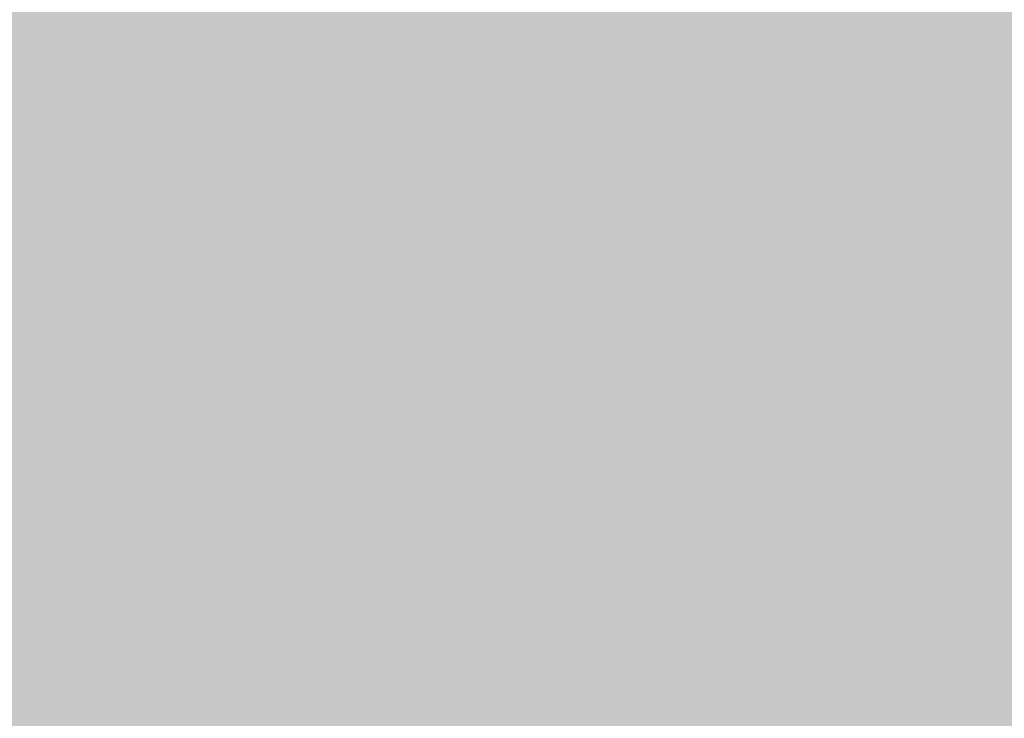
# Model space of a CAD drawing. Units: feet. Extents: x 3168 to 4724, y 827 to 1477.
# Tile 18 of 256: x 3257.497 to 3261.901, y 1093.654 to 1096.781. Entities that reach past the tile are written whole.
import ezdxf

# ---------------------------------------------------------------- set-up
doc = ezdxf.new("R2010")
doc.units = ezdxf.units.FT
doc.layers.add('A-ELEV-PATT', color=8, linetype='Continuous', lineweight=13)

msp = doc.modelspace()

# ---------------------------------------------------------------- hatches: boundary and pattern name
at = {"layer": 'A-ELEV-PATT'}
h = msp.add_hatch(color=256, dxfattribs=at)
h.dxf.hatch_style = 1
edge = h.paths.add_edge_path()
edge.add_ellipse((3552.9058, 979.2201), major_axis=(36.7449, 0), ratio=0.4848485, start_angle=0, end_angle=360)
edge = h.paths.add_edge_path()
edge.add_ellipse((3559.8916, 929.2523), major_axis=(36.7449, 0), ratio=0.4848485, start_angle=0, end_angle=360)
edge = h.paths.add_edge_path()
edge.add_line((3299.3168, 1198.6061), (3479.9167, 1198.6061))
edge.add_line((3479.9167, 1198.6061), (3479.9167, 1209.8686))
edge.add_spline(control_points=[(3479.9167, 1209.8686), (3464.3012, 1209.8686), (3448.6856, 1209.8686), (3410.9491, 1209.8686), (3388.8282, 1209.8686), (3355.6469, 1209.8686), (3344.5864, 1209.8686), (3327.9957, 1209.8686), (3322.4655, 1209.8686), (3314.1702, 1209.8686), (3311.4051, 1209.8686), (3307.2574, 1209.8686), (3305.8748, 1209.8686), (3303.801, 1209.8686), (3303.1097, 1209.8686), (3302.0728, 1209.8686), (3301.7272, 1209.8686), (3301.2087, 1209.8686), (3301.0359, 1209.8686), (3300.7767, 1209.8686), (3300.6903, 1209.8686), (3300.5606, 1209.8686), (3300.5174, 1209.8686), (3300.4526, 1209.8686), (3300.431, 1209.8686), (3300.3986, 1209.8686), (3300.3878, 1209.8686), (3300.3662, 1209.8686), (3300.3457, 1209.8686), (3300.3455, 1209.8686), (3300.3455, 1209.8686), (3300.3433, 1209.8686), (3300.3411, 1209.8686), (3300.3379, 1209.8686), (3300.3368, 1209.8686), (3300.3339, 1209.8686), (3300.3321, 1209.8686), (3300.3255, 1209.8686), (3300.3207, 1209.8686), (3300.3109, 1209.8686), (3300.306, 1209.8686), (3300.2905, 1209.8686), (3300.28, 1209.8686), (3300.2324, 1209.8688), (3300.1953, 1209.869), (3299.9511, 1209.8706), (3299.7448, 1209.8743), (3299.4368, 1209.8833), (3299.3344, 1209.8868), (3299.1811, 1209.8929), (3299.13, 1209.8951), (3298.6522, 1209.9168), (3298.2295, 1209.9457), (3297.6016, 1210.0024), (3297.3934, 1210.0235), (3297.0827, 1210.0583), (3296.9793, 1210.0705), (3296.293, 1210.1549), (3295.7181, 1210.2434), (3294.8687, 1210.3989), (3294.5877, 1210.4545), (3294.1693, 1210.5433), (3294.0304, 1210.5739), (3291.7071, 1211.1012), (3289.6536, 1211.8134), (3285.7763, 1213.564), (3283.9514, 1214.6035), (3280.5122, 1216.9801), (3278.8972, 1218.3176), (3276.3799, 1220.8295), (3275.416, 1221.9177), (3274.0393, 1223.7077), (3273.581, 1224.3495), (3273.1432, 1225.0163)], knot_values=[39.119033, 39.119033, 39.119033, 39.119033, 39.286353, 39.286353, 39.523379, 39.523379, 39.641892, 39.641892, 39.701148, 39.701148, 39.730777, 39.730777, 39.745591, 39.745591, 39.752998, 39.752998, 39.756701, 39.756701, 39.758553, 39.758553, 39.759479, 39.759479, 39.759942, 39.759942, 39.760173, 39.760173, 39.760289, 39.760289, 39.760405, 39.760405, 39.760463, 39.760463, 39.763389, 39.763389, 39.764851, 39.764851, 39.767304, 39.767304, 39.773825, 39.773825, 39.78057, 39.78057, 39.79477, 39.79477, 39.845194, 39.845194, 40.126715, 40.126715, 40.267476, 40.267476, 40.337856, 40.337856, 40.927023, 40.927023, 41.221606, 41.221606, 41.368898, 41.368898, 42.202622, 42.202622, 42.619485, 42.619485, 42.827916, 42.827916, 46.118323, 46.118323, 49.408731, 49.408731, 52.699139, 52.699139, 54.927489, 54.927489, 56.104228, 56.104228, 56.104228, 56.104228], weights=[1, 1, 1, 1, 1, 1, 1, 1, 1, 1, 1, 1, 1, 1, 1, 1, 1, 1, 1, 1, 1, 1, 1, 1, 1, 1, 1, 1, 1, 1, 1, 1, 1, 1, 1, 1, 1, 1, 1, 1, 1, 1, 1, 1, 1, 1, 1, 1, 1, 1, 1, 1, 1, 1, 1, 1, 1, 1, 1, 1, 1, 1, 1, 1, 1, 1, 1, 1, 1, 1, 1, 1, 1, 1], degree=3, periodic=0)
edge.add_line((3273.1432, 1225.0163), (3273.1432, 1099.0163))
edge.add_line((3273.1432, 1099.0163), (3299.3168, 1099.0163))
edge.add_line((3299.3168, 1099.0163), (3299.3168, 1198.6061))
edge = h.paths.add_edge_path()
edge.add_line((3304.7584, 1324.1581), (3479.9167, 1324.1581))
edge.add_line((3479.9167, 1324.1581), (3479.9167, 1335.7146))
edge.add_line((3479.9167, 1335.7146), (3269.1616, 1335.7146))
edge.add_spline(control_points=[(3269.1616, 1335.7146), (3264.0242, 1335.7146), (3258.3641, 1328.9582), (3259.2643, 1323.9003)], knot_values=[0, 0, 0, 0, 15.412191, 15.412191, 15.412191, 15.412191], degree=3, periodic=0)
edge.add_line((3259.2643, 1323.9003), (3265.5168, 1288.7691))
edge.add_line((3265.5168, 1288.7691), (3275.2651, 1261.5456))
edge.add_line((3275.2651, 1261.5456), (3304.7584, 1261.5456))
edge.add_line((3304.7584, 1261.5456), (3304.7584, 1324.1581))
h = msp.add_hatch(color=256, dxfattribs=at)
h.dxf.hatch_style = 1
h.paths.add_polyline_path([(3384.5252, 1099.0163), (3335.0292, 1099.0163), (3299.3168, 1099.0163), (3273.1432, 1099.0163), (3217.5654, 1099.0163), (3168.0693, 827.1163), (3335.0292, 827.1163)])

doc.saveas('drawing.dxf')
